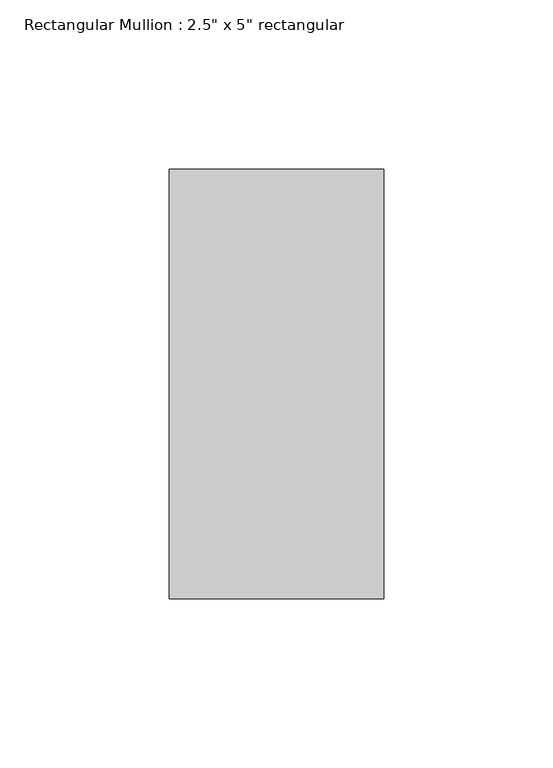
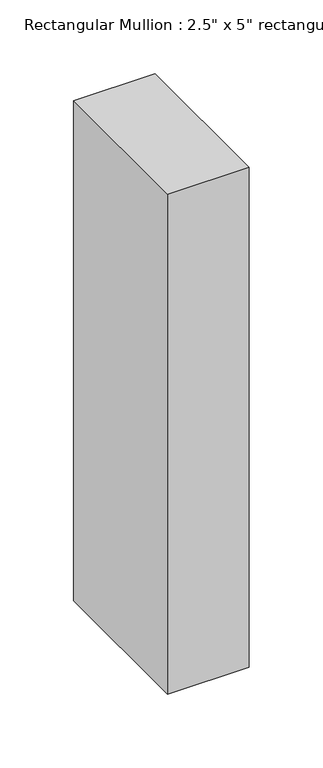
"""IFC4 building model written with IfcOpenShell, lengths in millimetres: member geometry."""

from ifc_helpers import new_model, si_unit, frame, origin, place, context, project, spatial, polyline, outline, extrude, source, transform, mapped, element, save


def member_dc106669(model_context):
    return source(origin(), model_context, "Body", "SweptSolid", [
        extrude(outline(polyline([(0.0, 63.5), (0.0, -63.5), (-63.5, -63.5), (-63.5, 63.5), (0.0, 63.5)])), frame((0.0, 0.0, -412.75), z_axis=(0.0, 0.0, 1.0), x_axis=(1.0, 0.0, 0.0)), (0.0, 0.0, 1.0), 412.75),
    ])


if __name__ == "__main__":
    model = new_model("IFC4")
    model_context = context("Model", 3, world=origin())
    ifc_project = project(units=[si_unit("LENGTHUNIT", "METRE", prefix="MILLI")], contexts=[model_context])
    site = spatial("IfcSite", under=ifc_project)
    building = spatial("IfcBuilding", under=site)
    placement = place(None, origin())
    member_shape = member_dc106669(model_context)
    element("IfcMember", 1, ObjectType="Rectangular Mullion : 2.5\" x 5\" rectangular", at=placement, inside=building, context=model_context, shape_type="MappedRepresentation", body=[
        mapped(member_shape, transform((0.0, 0.0, 0.0), x_axis=(1.0, 0.0, 0.0), y_axis=(0.0, 1.0, 0.0), z_axis=(0.0, 0.0, 1.0))),
    ])
    save(model, "model.ifc")

# Revit data of these elements
# Type "Rectangular Mullion : 2.5\" x 5\" rectangular"
#   built-in parameter 1007304 = 0.416667 (stored number, unit not read)
#   built-in parameter 1007301 = 0.104167 (stored number, unit not read)
#   built-in parameter 1007300 = 0.104167 (stored number, unit not read)
# Element 1 (IfcMember, "Rectangular Mullion : 2.5\" x 5\" rectangular")
#   Materials on its faces: "Aluminum"
# Materials
#   "Aluminum": class "Metal", colour RGB 247 247 247, transparency 0, Description = "Aluminum 6061", Cost = 0
